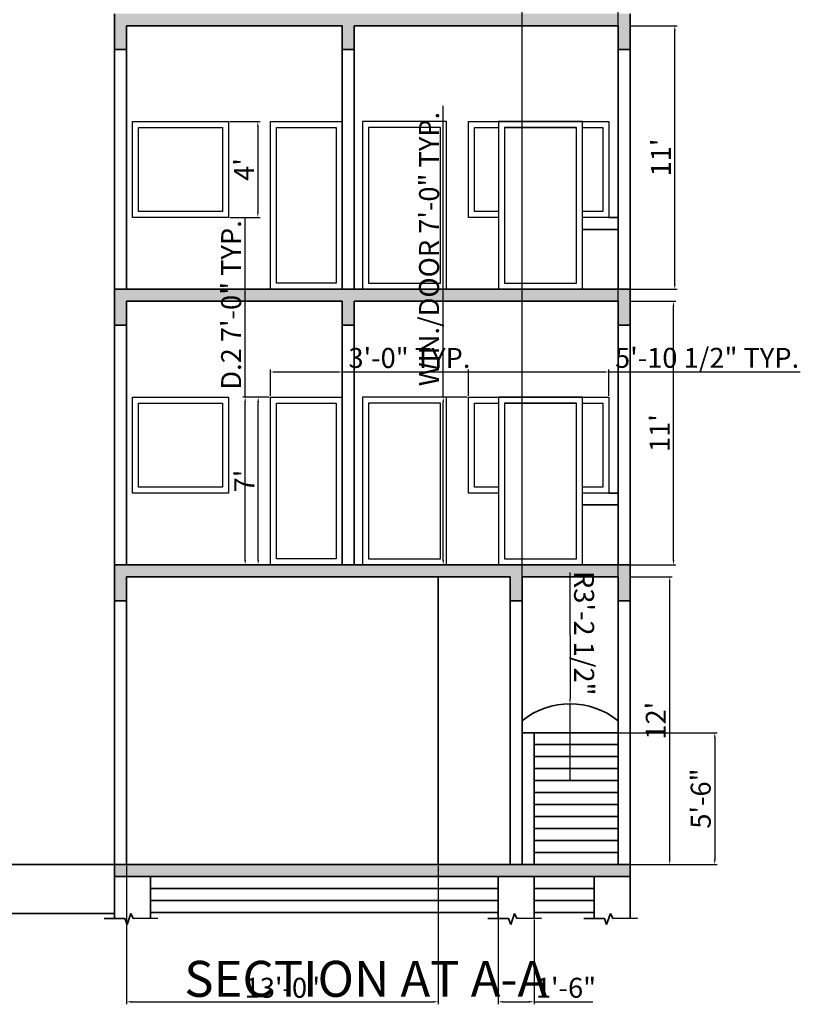
# Model space of a CAD drawing. Units: inches. Extents: x 2368 to 3882, y 1243 to 2139.
# Tile 5 of 6: x 3491 to 3882, y 1252 to 1745. Entities that reach past the tile are written whole.
import ezdxf

# ---------------------------------------------------------------- set-up
doc = ezdxf.new("R2010")
doc.units = ezdxf.units.IN
for name, color, linetype, lineweight in [('A-ANNO-DIMS', 2, 'Continuous', 18), ('A-ANNO-TEXT', 7, 'Continuous', 18), ('A-ELEV', 7, 'Continuous', 25), ('A-SECT', 7, 'Continuous', 35), ('A-SECT-PATT', 8, 'Continuous', 13)]:
    doc.layers.add(name, color=color, linetype=linetype, lineweight=lineweight)
doc.styles.get("Standard").update_dxf_attribs({"font": 'arial.ttf'})
doc.dimstyles.new('ISO-25', dxfattribs={"dimtxt": 10, "dimasz": 2.5, "dimexe": 1.25, "dimexo": 0.625, "dimtad": 1, "dimlunit": 3, "dimtxsty": 'Standard', "dimcen": 2.5, "dimadec": 0, "dimazin": 0, "dimtfac": 1, "dimtmove": 0, "dimatfit": 3, "dimfxl": 1, "dimarcsym": 0})

# ---------------------------------------------------------------- blocks, each defined once
blk = doc.blocks.new('*D8')
at = {"layer": 'A-ANNO-DIMS', "color": 0, "lineweight": -2, "transparency": 16777216}
for p, q in [((3615.71, 1555.84), (3609, 1555.84)), ((3610.25, 1474.34), (3610.25, 1553.34)), ((3615.71, 1471.84), (3609, 1471.84))]:
    blk.add_line(p, q, dxfattribs=at)
at = {"layer": 'A-ANNO-DIMS', "color": 0, "transparency": 16777216}
for points in [[(3609.83, 1553.34), (3610.67, 1553.34), (3610.25, 1555.84)], [(3609.83, 1474.34), (3610.67, 1474.34), (3610.25, 1471.84)]]:
    blk.add_solid(points, dxfattribs=at)
at = {"layer": 'Defpoints', "color": 0, "transparency": 16777216}
for p in [(3610.25, 1555.84), (3616.34, 1555.84), (3616.34, 1471.84)]:
    blk.add_point(p, dxfattribs=at)
at = {"layer": 'A-ANNO-DIMS', "color": 0, "transparency": 16777216, "insert": (3604.62, 1513.84), "char_height": 10, "attachment_point": 5, "rotation": 90}
blk.add_mtext("7'", dxfattribs=at)
blk = doc.blocks.new('*D9')
at = {"layer": 'A-ANNO-DIMS', "color": 0, "lineweight": -2, "transparency": 16777216}
for p, q in [((3596.02, 1693.84), (3611.32, 1693.84)), ((3610.07, 1691.34), (3610.07, 1648.34)), ((3596.02, 1645.84), (3611.32, 1645.84))]:
    blk.add_line(p, q, dxfattribs=at)
at = {"layer": 'A-ANNO-DIMS', "color": 0, "transparency": 16777216}
for points in [[(3609.65, 1691.34), (3610.48, 1691.34), (3610.07, 1693.84)], [(3609.65, 1648.34), (3610.48, 1648.34), (3610.07, 1645.84)]]:
    blk.add_solid(points, dxfattribs=at)
at = {"layer": 'Defpoints', "color": 0, "transparency": 16777216}
for p in [(3595.39, 1693.84), (3595.39, 1645.84), (3610.07, 1645.84)]:
    blk.add_point(p, dxfattribs=at)
at = {"layer": 'A-ANNO-DIMS', "color": 0, "transparency": 16777216, "insert": (3604.44, 1669.84), "char_height": 10, "attachment_point": 5, "rotation": 90}
blk.add_mtext("4'", dxfattribs=at)
blk = doc.blocks.new('*D10')
at = {"layer": 'A-ANNO-DIMS', "color": 0, "lineweight": -2, "transparency": 16777216}
for p, q in [((3796.96, 1465.84), (3817.44, 1465.84)), ((3816.19, 1324.34), (3816.19, 1463.34)), ((3796.96, 1321.84), (3817.44, 1321.84))]:
    blk.add_line(p, q, dxfattribs=at)
at = {"layer": 'A-ANNO-DIMS', "color": 0, "transparency": 16777216}
for points in [[(3815.77, 1463.34), (3816.6, 1463.34), (3816.19, 1465.84)], [(3815.77, 1324.34), (3816.6, 1324.34), (3816.19, 1321.84)]]:
    blk.add_solid(points, dxfattribs=at)
at = {"layer": 'Defpoints', "color": 0, "transparency": 16777216}
for p in [(3796.34, 1465.84), (3816.19, 1465.84), (3796.34, 1321.84)]:
    blk.add_point(p, dxfattribs=at)
at = {"layer": 'A-ANNO-DIMS', "color": 0, "transparency": 16777216, "insert": (3810.54, 1393.84), "char_height": 10, "attachment_point": 5, "rotation": 90}
blk.add_mtext("12'", dxfattribs=at)
blk = doc.blocks.new('*D11')
at = {"layer": 'A-ANNO-DIMS', "color": 0, "lineweight": -2, "transparency": 16777216}
for p, q in [((3796.96, 1603.84), (3819.34, 1603.84)), ((3818.09, 1474.34), (3818.09, 1601.34)), ((3796.96, 1471.84), (3819.34, 1471.84))]:
    blk.add_line(p, q, dxfattribs=at)
at = {"layer": 'A-ANNO-DIMS', "color": 0, "transparency": 16777216}
for points in [[(3817.68, 1601.34), (3818.51, 1601.34), (3818.09, 1603.84)], [(3817.68, 1474.34), (3818.51, 1474.34), (3818.09, 1471.84)]]:
    blk.add_solid(points, dxfattribs=at)
at = {"layer": 'Defpoints', "color": 0, "transparency": 16777216}
for p in [(3796.34, 1603.84), (3818.09, 1603.84), (3796.34, 1471.84)]:
    blk.add_point(p, dxfattribs=at)
at = {"layer": 'A-ANNO-DIMS', "color": 0, "transparency": 16777216, "insert": (3812.45, 1537.84), "char_height": 10, "attachment_point": 5, "rotation": 90}
blk.add_mtext("11'", dxfattribs=at)
blk = doc.blocks.new('*D12')
at = {"layer": 'A-ANNO-DIMS', "color": 0, "lineweight": -2, "transparency": 16777216}
for p, q in [((3796.96, 1741.84), (3819.98, 1741.84)), ((3818.73, 1612.34), (3818.73, 1739.34)), ((3796.96, 1609.84), (3819.98, 1609.84))]:
    blk.add_line(p, q, dxfattribs=at)
at = {"layer": 'A-ANNO-DIMS', "color": 0, "transparency": 16777216}
for points in [[(3818.31, 1739.34), (3819.15, 1739.34), (3818.73, 1741.84)], [(3818.31, 1612.34), (3819.15, 1612.34), (3818.73, 1609.84)]]:
    blk.add_solid(points, dxfattribs=at)
at = {"layer": 'Defpoints', "color": 0, "transparency": 16777216}
for p in [(3796.34, 1741.84), (3818.73, 1741.84), (3796.34, 1609.84)]:
    blk.add_point(p, dxfattribs=at)
at = {"layer": 'A-ANNO-DIMS', "color": 0, "transparency": 16777216, "insert": (3813.09, 1675.84), "char_height": 10, "attachment_point": 5, "rotation": 90}
blk.add_mtext("11'", dxfattribs=at)
blk = doc.blocks.new('WIN-SECT-SQ')
for points in [[(3547.39, 1831.84), (3595.39, 1831.84), (3595.39, 1783.84), (3547.39, 1783.84)], [(3550.39, 1828.84), (3592.39, 1828.84), (3592.39, 1786.84), (3550.39, 1786.84)]]:
    blk.add_lwpolyline(points, close=True)
blk = doc.blocks.new('DOOR-SECT')
for points in [[(3662.52, 1747.84), (3704.52, 1747.84), (3704.52, 1831.84), (3662.52, 1831.84)], [(3665.52, 1750.84), (3701.52, 1750.84), (3701.52, 1828.84), (3665.52, 1828.84)]]:
    blk.add_lwpolyline(points, close=True)
blk = doc.blocks.new('DOOR-SECT-2')
for points in [[(3652.34, 1471.84), (3616.34, 1471.84), (3616.34, 1555.84), (3652.34, 1555.84)], [(3649.34, 1474.84), (3619.34, 1474.84), (3619.34, 1552.84), (3649.34, 1552.84)]]:
    blk.add_lwpolyline(points, close=True)
blk = doc.blocks.new('WIN-DOOR-SECT')
for points in [[(3730.54, 1783.84), (3715.45, 1783.84), (3715.45, 1831.84), (3785.77, 1831.84), (3785.77, 1783.84), (3772.54, 1783.84)], [(3730.54, 1786.84), (3718.45, 1786.84), (3718.45, 1828.84), (3730.54, 1828.84)], [(3733.54, 1828.84), (3769.54, 1828.84)], [(3772.54, 1828.84), (3782.77, 1828.84), (3782.77, 1786.84), (3772.54, 1786.84)]]:
    blk.add_lwpolyline(points)
for points in [[(3730.54, 1747.84), (3772.54, 1747.84), (3772.54, 1831.84), (3730.54, 1831.84)], [(3733.54, 1750.84), (3769.54, 1750.84), (3769.54, 1828.84), (3733.54, 1828.84)]]:
    blk.add_lwpolyline(points, close=True)
blk = doc.blocks.new('*D24')
at = {"layer": 'A-ANNO-DIMS', "color": 0, "lineweight": -2, "transparency": 16777216}
for p, q in [((3702.85, 1555.84), (3702.85, 1701.66)), ((3714.83, 1555.84), (3701.6, 1555.84)), ((3702.85, 1474.34), (3702.85, 1553.34)), ((3714.83, 1471.84), (3701.6, 1471.84))]:
    blk.add_line(p, q, dxfattribs=at)
at = {"layer": 'A-ANNO-DIMS', "color": 0, "transparency": 16777216}
for points in [[(3702.44, 1553.34), (3703.27, 1553.34), (3702.85, 1555.84)], [(3702.44, 1474.34), (3703.27, 1474.34), (3702.85, 1471.84)]]:
    blk.add_solid(points, dxfattribs=at)
at = {"layer": 'Defpoints', "color": 0, "transparency": 16777216}
for p in [(3702.85, 1555.84), (3715.45, 1555.84), (3715.45, 1471.84)]:
    blk.add_point(p, dxfattribs=at)
at = {"layer": 'A-ANNO-DIMS', "color": 0, "transparency": 16777216, "insert": (3697.06, 1630), "char_height": 10, "attachment_point": 5, "rotation": 90}
blk.add_mtext('WIN./DOOR 7\'-0" TYP.', dxfattribs=at)
blk = doc.blocks.new('*D25')
at = {"layer": 'A-ANNO-DIMS', "color": 0, "lineweight": -2, "transparency": 16777216}
for p, q in [((3715.45, 1556.46), (3715.45, 1569.69)), ((3717.95, 1568.44), (3783.27, 1568.44)), ((3785.77, 1556.46), (3785.77, 1569.69)), ((3785.77, 1568.44), (3881.55, 1568.44))]:
    blk.add_line(p, q, dxfattribs=at)
at = {"layer": 'A-ANNO-DIMS', "color": 0, "transparency": 16777216}
for points in [[(3717.95, 1568.85), (3717.95, 1568.02), (3715.45, 1568.44)], [(3783.27, 1568.85), (3783.27, 1568.02), (3785.77, 1568.44)]]:
    blk.add_solid(points, dxfattribs=at)
at = {"layer": 'Defpoints', "color": 0, "transparency": 16777216}
for p in [(3785.77, 1568.44), (3715.45, 1555.84), (3785.77, 1555.84)]:
    blk.add_point(p, dxfattribs=at)
at = {"layer": 'A-ANNO-DIMS', "color": 0, "transparency": 16777216, "insert": (3834.91, 1574.23), "char_height": 10, "attachment_point": 5}
blk.add_mtext('5\'-10 1/2" TYP.', dxfattribs=at)
blk = doc.blocks.new('*D30')
at = {"layer": 'A-ANNO-DIMS', "color": 0, "lineweight": -2, "transparency": 16777216}
for p, q in [((3603.74, 1555.84), (3603.74, 1645.67)), ((3615.71, 1555.84), (3602.49, 1555.84)), ((3603.74, 1474.34), (3603.74, 1553.34)), ((3615.71, 1471.84), (3602.49, 1471.84))]:
    blk.add_line(p, q, dxfattribs=at)
at = {"layer": 'A-ANNO-DIMS', "color": 0, "transparency": 16777216}
for points in [[(3603.32, 1553.34), (3604.15, 1553.34), (3603.74, 1555.84)], [(3603.32, 1474.34), (3604.15, 1474.34), (3603.74, 1471.84)]]:
    blk.add_solid(points, dxfattribs=at)
at = {"layer": 'Defpoints', "color": 0, "transparency": 16777216}
for p in [(3603.74, 1555.84), (3616.34, 1555.84), (3616.34, 1471.84)]:
    blk.add_point(p, dxfattribs=at)
at = {"layer": 'A-ANNO-DIMS', "color": 0, "transparency": 16777216, "insert": (3598.01, 1602), "char_height": 10, "attachment_point": 5, "rotation": 90}
blk.add_mtext('D.2 7\'-0" TYP.', dxfattribs=at)
blk = doc.blocks.new('*D31')
at = {"layer": 'A-ANNO-DIMS', "color": 0, "lineweight": -2, "transparency": 16777216}
for p, q in [((3616.34, 1556.46), (3616.34, 1569.69)), ((3618.84, 1568.44), (3649.84, 1568.44)), ((3652.34, 1556.46), (3652.34, 1569.69)), ((3652.34, 1568.44), (3717.04, 1568.44))]:
    blk.add_line(p, q, dxfattribs=at)
at = {"layer": 'A-ANNO-DIMS', "color": 0, "transparency": 16777216}
for points in [[(3618.84, 1568.85), (3618.84, 1568.02), (3616.34, 1568.44)], [(3649.84, 1568.85), (3649.84, 1568.02), (3652.34, 1568.44)]]:
    blk.add_solid(points, dxfattribs=at)
at = {"layer": 'Defpoints', "color": 0, "transparency": 16777216}
for p in [(3652.34, 1568.44), (3616.34, 1555.84), (3652.34, 1555.84)]:
    blk.add_point(p, dxfattribs=at)
at = {"layer": 'A-ANNO-DIMS', "color": 0, "transparency": 16777216, "insert": (3685.94, 1574.17), "char_height": 10, "attachment_point": 5}
blk.add_mtext('3\'-0" TYP.', dxfattribs=at)
blk = doc.blocks.new('*D92')
at = {"layer": 'A-ANNO-DIMS', "color": 0, "lineweight": -2, "transparency": 16777216}
for p, q in [((3380.64, 1321.84), (3380.64, 1375.64)), ((3537.71, 1321.84), (3379.39, 1321.84)), ((3380.64, 1299.76), (3380.64, 1319.34)), ((3537.71, 1297.26), (3379.39, 1297.26))]:
    blk.add_line(p, q, dxfattribs=at)
at = {"layer": 'A-ANNO-DIMS', "color": 0, "transparency": 16777216}
for points in [[(3380.23, 1319.34), (3381.06, 1319.34), (3380.64, 1321.84)], [(3380.23, 1299.76), (3381.06, 1299.76), (3380.64, 1297.26)]]:
    blk.add_solid(points, dxfattribs=at)
at = {"layer": 'Defpoints', "color": 0, "transparency": 16777216}
for p in [(3380.64, 1321.84), (3538.34, 1321.84), (3538.34, 1297.26)]:
    blk.add_point(p, dxfattribs=at)
at = {"layer": 'A-ANNO-DIMS', "color": 0, "transparency": 16777216, "insert": (3374.85, 1349.99), "char_height": 10, "attachment_point": 5, "rotation": 90}
blk.add_mtext('2\'-0 1/2"', dxfattribs=at)
blk = doc.blocks.new('*D93')
at = {"layer": 'A-ANNO-DIMS', "color": 0, "lineweight": -2, "transparency": 16777216}
for p, q in [((3730.34, 1294.21), (3730.34, 1251.83)), ((3748.34, 1294.21), (3748.34, 1251.83)), ((3732.84, 1253.08), (3745.84, 1253.08)), ((3748.34, 1253.08), (3777.73, 1253.08))]:
    blk.add_line(p, q, dxfattribs=at)
at = {"layer": 'A-ANNO-DIMS', "color": 0, "transparency": 16777216}
for points in [[(3732.84, 1253.49), (3732.84, 1252.66), (3730.34, 1253.08)], [(3745.84, 1253.49), (3745.84, 1252.66), (3748.34, 1253.08)]]:
    blk.add_solid(points, dxfattribs=at)
at = {"layer": 'Defpoints', "color": 0, "transparency": 16777216}
for p in [(3730.34, 1294.84), (3748.34, 1294.84), (3748.34, 1253.08)]:
    blk.add_point(p, dxfattribs=at)
at = {"layer": 'A-ANNO-DIMS', "color": 0, "transparency": 16777216, "insert": (3764.28, 1258.81), "char_height": 10, "attachment_point": 5}
blk.add_mtext('1\'-6"', dxfattribs=at)
blk = doc.blocks.new('*D94')
at = {"layer": 'A-ANNO-DIMS', "color": 0, "lineweight": -2, "transparency": 16777216}
for p, q in [((3742.34, 1388.46), (3742.34, 2045.79)), ((3744.84, 2044.54), (3787.84, 2044.54)), ((3790.34, 1388.46), (3790.34, 2045.79))]:
    blk.add_line(p, q, dxfattribs=at)
at = {"layer": 'A-ANNO-DIMS', "color": 0, "transparency": 16777216}
for points in [[(3744.84, 2044.95), (3744.84, 2044.12), (3742.34, 2044.54)], [(3787.84, 2044.95), (3787.84, 2044.12), (3790.34, 2044.54)]]:
    blk.add_solid(points, dxfattribs=at)
at = {"layer": 'Defpoints', "color": 0, "transparency": 16777216}
for p in [(3790.34, 2044.54), (3742.34, 1387.84), (3790.34, 1387.84)]:
    blk.add_point(p, dxfattribs=at)
at = {"layer": 'A-ANNO-DIMS', "color": 0, "transparency": 16777216, "insert": (3766.34, 2050.27), "char_height": 10, "attachment_point": 5}
blk.add_mtext('4\'-0"', dxfattribs=at)
blk = doc.blocks.new('*D95')
at = {"layer": 'A-ANNO-DIMS', "color": 0, "lineweight": -2, "transparency": 16777216}
for p, q in [((3790.96, 1387.84), (3839.99, 1387.84)), ((3838.74, 1385.34), (3838.74, 1324.34)), ((3790.96, 1321.84), (3839.99, 1321.84))]:
    blk.add_line(p, q, dxfattribs=at)
at = {"layer": 'A-ANNO-DIMS', "color": 0, "transparency": 16777216}
for points in [[(3838.33, 1385.34), (3839.16, 1385.34), (3838.74, 1387.84)], [(3838.33, 1324.34), (3839.16, 1324.34), (3838.74, 1321.84)]]:
    blk.add_solid(points, dxfattribs=at)
at = {"layer": 'Defpoints', "color": 0, "transparency": 16777216}
for p in [(3790.34, 1387.84), (3790.34, 1321.84), (3838.74, 1321.84)]:
    blk.add_point(p, dxfattribs=at)
at = {"layer": 'A-ANNO-DIMS', "color": 0, "transparency": 16777216, "insert": (3833.01, 1354.84), "char_height": 10, "attachment_point": 5, "rotation": 90}
blk.add_mtext('5\'-6"', dxfattribs=at)
blk = doc.blocks.new('*D96')
at = {"layer": 'A-ANNO-DIMS', "color": 0, "lineweight": -2, "transparency": 16777216}
for p, q in [((3544.34, 1321.21), (3544.34, 1251.83)), ((3700.34, 1321.21), (3700.34, 1251.83)), ((3546.84, 1253.08), (3697.84, 1253.08))]:
    blk.add_line(p, q, dxfattribs=at)
at = {"layer": 'A-ANNO-DIMS', "color": 0, "transparency": 16777216}
for points in [[(3546.84, 1253.49), (3546.84, 1252.66), (3544.34, 1253.08)], [(3697.84, 1253.49), (3697.84, 1252.66), (3700.34, 1253.08)]]:
    blk.add_solid(points, dxfattribs=at)
at = {"layer": 'Defpoints', "color": 0, "transparency": 16777216}
for p in [(3544.34, 1321.84), (3700.34, 1321.84), (3700.34, 1253.08)]:
    blk.add_point(p, dxfattribs=at)
at = {"layer": 'A-ANNO-DIMS', "color": 0, "transparency": 16777216, "insert": (3622.34, 1258.81), "char_height": 10, "attachment_point": 5}
blk.add_mtext('13\'-0"', dxfattribs=at)
blk = doc.blocks.new('*D98')
at = {"layer": 'A-ANNO-DIMS', "color": 0, "lineweight": -2, "transparency": 16777216}
for p, q in [((3766.24, 1467.96), (3766.3, 1404.76)), ((3766.34, 1363.84), (3766.3, 1402.26))]:
    blk.add_line(p, q, dxfattribs=at)
at = {"layer": 'A-ANNO-DIMS', "color": 0, "transparency": 16777216}
blk.add_solid([(3766.71, 1404.76), (3765.88, 1404.76), (3766.3, 1402.26)], dxfattribs=at)
at = {"layer": 'Defpoints', "color": 0, "transparency": 16777216}
for p in [(3766.3, 1402.26), (3766.34, 1363.84)]:
    blk.add_point(p, dxfattribs=at)
at = {"layer": 'A-ANNO-DIMS', "color": 0, "transparency": 16777216, "insert": (3772.06, 1437.61), "char_height": 10, "attachment_point": 5, "rotation": 270.0563}
blk.add_mtext('R3\'-2 1/2"', dxfattribs=at)

msp = doc.modelspace()

# ---------------------------------------------------------------- hatches: boundary and pattern name
at = {"layer": 'A-SECT-PATT'}
h = msp.add_hatch(color=256, dxfattribs=at)
h.dxf.hatch_style = 1
h.paths.add_polyline_path([(3796.338, 1321.838), (3538.338, 1321.838), (3538.338, 1315.838), (3796.338, 1315.838)])
h.paths.add_polyline_path([(3796.338, 1471.838), (3538.338, 1471.838), (3538.338, 1453.838), (3544.338, 1453.838), (3544.338, 1465.838), (3736.338, 1465.838), (3736.338, 1453.838), (3742.338, 1453.838), (3742.338, 1465.838), (3790.338, 1465.838), (3790.338, 1453.838), (3796.338, 1453.838), (3796.338, 1465.838)])
h.paths.add_polyline_path([(3796.338, 1609.838), (3538.338, 1609.838), (3538.338, 1591.838), (3544.338, 1591.838), (3544.338, 1603.838), (3652.338, 1603.838), (3652.338, 1591.838), (3658.338, 1591.838), (3658.338, 1603.838), (3790.338, 1603.838), (3790.338, 1591.838), (3796.338, 1591.838), (3796.338, 1603.838)])
h.paths.add_polyline_path([(3796.338, 1747.838), (3538.338, 1747.838), (3538.338, 1729.838), (3544.338, 1729.838), (3544.338, 1741.838), (3652.338, 1741.838), (3652.338, 1729.838), (3658.338, 1729.838), (3658.338, 1741.838), (3790.338, 1741.838), (3790.338, 1729.838), (3796.338, 1729.838), (3796.338, 1741.838)])
h.paths.add_polyline_path([(3796.338, 1885.838), (3538.338, 1885.838), (3538.338, 1867.838), (3544.338, 1867.838), (3544.338, 1879.838), (3652.338, 1879.838), (3652.338, 1867.838), (3658.338, 1867.838), (3658.338, 1879.838), (3790.338, 1879.838), (3790.338, 1867.838), (3796.338, 1867.838), (3796.338, 1879.838)])

# ---------------------------------------------------------------- linework, layer by layer
at = {"layer": 'A-SECT'}
for p, q in [((3538.338, 1609.838), (3538.338, 1747.838)), ((3796.338, 1741.838), (3796.338, 1747.838)), ((3544.338, 1741.838), (3652.338, 1741.838)), ((3544.338, 1609.838), (3544.338, 1741.838)), ((3652.338, 1609.838), (3652.338, 1741.838)), ((3658.338, 1609.838), (3658.338, 1741.838)), ((3658.338, 1741.838), (3790.338, 1741.838)), ((3790.338, 1609.838), (3790.338, 1741.838)), ((3796.338, 1609.838), (3796.338, 1741.838)), ((3544.338, 1729.838), (3538.338, 1729.838)), ((3658.338, 1729.838), (3652.338, 1729.838)), ((3796.338, 1729.838), (3790.338, 1729.838)), ((3785.773, 1645.838), (3790.338, 1645.838)), ((3772.538, 1639.838), (3790.338, 1639.838)), ((3538.338, 1471.838), (3538.338, 1609.838)), ((3796.338, 1609.838), (3538.338, 1609.838)), ((3796.338, 1603.838), (3796.338, 1609.838)), ((3544.338, 1603.838), (3652.338, 1603.838)), ((3544.338, 1471.838), (3544.338, 1603.838)), ((3652.338, 1471.838), (3652.338, 1603.838)), ((3658.338, 1471.838), (3658.338, 1603.838)), ((3658.338, 1603.838), (3790.338, 1603.838)), ((3790.338, 1471.838), (3790.338, 1603.838)), ((3796.338, 1471.838), (3796.338, 1603.838)), ((3544.338, 1591.838), (3538.338, 1591.838)), ((3658.338, 1591.838), (3652.338, 1591.838)), ((3796.338, 1591.838), (3790.338, 1591.838)), ((3785.773, 1507.838), (3790.338, 1507.838)), ((3772.538, 1501.838), (3790.338, 1501.838)), ((3538.338, 1294.838), (3538.338, 1471.838)), ((3796.338, 1471.838), (3538.338, 1471.838)), ((3796.338, 1465.838), (3796.338, 1471.838)), ((3544.338, 1465.838), (3736.338, 1465.838)), ((3544.338, 1321.838), (3544.338, 1465.838)), ((3700.338, 1321.838), (3700.338, 1465.838)), ((3736.338, 1321.838), (3736.338, 1465.838)), ((3742.338, 1321.838), (3742.338, 1465.838)), ((3742.338, 1465.838), (3790.338, 1465.838)), ((3790.338, 1321.838), (3790.338, 1465.838)), ((3796.338, 1321.838), (3796.338, 1465.838)), ((3544.338, 1453.838), (3538.338, 1453.838)), ((3742.338, 1453.838), (3736.338, 1453.838)), ((3796.338, 1453.838), (3790.338, 1453.838)), ((3790.338, 1387.838), (3742.338, 1387.838)), ((3748.338, 1321.838), (3748.338, 1387.838)), ((3790.338, 1381.838), (3748.338, 1381.838)), ((3790.338, 1375.838), (3748.338, 1375.838)), ((3790.338, 1369.838), (3748.338, 1369.838)), ((3790.338, 1363.838), (3748.338, 1363.838)), ((3790.338, 1357.838), (3748.338, 1357.838)), ((3790.338, 1351.838), (3748.338, 1351.838)), ((3790.338, 1345.838), (3748.338, 1345.838)), ((3790.338, 1339.838), (3748.338, 1339.838)), ((3790.338, 1333.838), (3748.338, 1333.838)), ((3790.338, 1327.838), (3748.338, 1327.838)), ((3538.338, 1321.838), (3419.342, 1321.838)), ((3796.338, 1321.838), (3538.338, 1321.838)), ((3790.338, 1321.838), (3742.338, 1321.838)), ((3796.338, 1294.838), (3796.338, 1321.838)), ((3796.338, 1315.838), (3538.338, 1315.838)), ((3556.338, 1294.838), (3556.338, 1315.838)), ((3730.338, 1294.838), (3730.338, 1315.838)), ((3748.338, 1294.838), (3748.338, 1315.838)), ((3778.338, 1294.838), (3778.338, 1315.838)), ((3730.338, 1309.838), (3556.338, 1309.838)), ((3778.338, 1309.838), (3748.338, 1309.838)), ((3730.338, 1303.838), (3556.338, 1303.838)), ((3778.338, 1303.838), (3748.338, 1303.838)), ((3538.338, 1297.261), (3420.08, 1297.261)), ((3544.63, 1291.775), (3546.535, 1297.313)), ((3546.535, 1297.313), (3547.712, 1294.838)), ((3556.338, 1297.838), (3730.338, 1297.838)), ((3736.63, 1291.775), (3738.535, 1297.313)), ((3738.535, 1297.313), (3739.712, 1294.838)), ((3748.338, 1297.838), (3778.338, 1297.838)), ((3784.63, 1291.775), (3786.535, 1297.313)), ((3786.535, 1297.313), (3787.712, 1294.838)), ((3533.199, 1294.838), (3543.486, 1294.838)), ((3543.486, 1294.838), (3544.63, 1291.775)), ((3547.712, 1294.838), (3560.044, 1294.89)), ((3725.199, 1294.838), (3735.486, 1294.838)), ((3735.486, 1294.838), (3736.63, 1291.775)), ((3739.712, 1294.838), (3752.044, 1294.89)), ((3773.199, 1294.838), (3783.486, 1294.838)), ((3783.486, 1294.838), (3784.63, 1291.775)), ((3787.712, 1294.838), (3800.044, 1294.89))]:
    msp.add_line(p, q, dxfattribs=at)
msp.add_arc((3766.338, 1363.838), 38.419, 51.34019, 128.65981, dxfattribs=at)

# ---------------------------------------------------------------- block references
at = {"layer": 'A-ELEV'}
for name, p in [('WIN-SECT-SQ', (0, -138)), ('DOOR-SECT-2', (0, 138)), ('DOOR-SECT', (0, -138)), ('WIN-DOOR-SECT', (0, -138)), ('WIN-SECT-SQ', (0, -276)), ('DOOR-SECT-2', (0, 0)), ('DOOR-SECT', (0, -276)), ('WIN-DOOR-SECT', (0, -276))]:
    msp.add_blockref(name, p, dxfattribs=at)

# ---------------------------------------------------------------- texts
at = {"layer": 'A-ANNO-TEXT'}
msp.add_text('SECTION AT A-A', height=18, dxfattribs=at).set_placement((3573.285, 1255.58))

# ---------------------------------------------------------------- dimensions: what is measured, and where the dimension line sits
at = {"layer": 'A-ANNO-DIMS'}
for base, p1, p2, picture, middle in [((3790.338, 2044.538), (3742.338, 1387.838), (3790.338, 1387.838), '*D94', (3766.338, 2050.268)), ((3700.338, 1253.075), (3544.338, 1321.838), (3700.338, 1321.838), '*D96', (3622.338, 1258.809)), ((3748.338, 1253.075), (3730.338, 1294.838), (3748.338, 1294.838), '*D93', (3764.283, 1258.806))]:
    dim = msp.add_linear_dim(base=base, p1=p1, p2=p2, dimstyle='ISO-25', override={"dimdec": 1, "dimlfac": 1, "dimrnd": 0, "dimzin": 1, "dimdsep": 46, "dimlunit": 4, "dimfrac": 2}, dxfattribs=at)
    dim.commit()
    dim.dimension.update_dxf_attribs({"geometry": picture, "text_midpoint": middle})
for base, p1, p2, override, picture, middle in [((3818.731, 1741.838), (3796.338, 1609.838), (3796.338, 1741.838), {"dimclrd": 0, "dimclre": 0, "dimclrt": 0}, '*D12', (3813.086, 1675.838)), ((3610.065, 1645.838), (3595.393, 1693.838), (3595.393, 1645.838), {"dimclrd": 0, "dimclre": 0, "dimclrt": 0}, '*D9', (3604.44, 1669.838)), ((3818.095, 1603.838), (3796.338, 1471.838), (3796.338, 1603.838), {"dimclrd": 0, "dimclre": 0, "dimclrt": 0}, '*D11', (3812.449, 1537.838)), ((3610.25, 1555.838), (3616.338, 1471.838), (3616.338, 1555.838), {"dimclrd": 0, "dimclre": 0, "dimclrt": 0}, '*D8', (3604.625, 1513.838)), ((3816.188, 1465.838), (3796.338, 1321.838), (3796.338, 1465.838), {"dimclrd": 0, "dimclre": 0, "dimclrt": 0}, '*D10', (3810.543, 1393.838)), ((3838.744, 1321.838), (3790.338, 1387.838), (3790.338, 1321.838), {"dimdec": 1, "dimlfac": 1, "dimrnd": 0, "dimzin": 1, "dimdsep": 46, "dimlunit": 4, "dimfrac": 2}, '*D95', (3833.013, 1354.838)), ((3380.642, 1321.838), (3538.338, 1297.261), (3538.338, 1321.838), {"dimdec": 1, "dimlfac": 1, "dimrnd": 0, "dimzin": 1, "dimdsep": 46, "dimlunit": 4, "dimfrac": 2}, '*D92', (3374.847, 1349.99))]:
    dim = msp.add_linear_dim(base=base, p1=p1, p2=p2, angle=90, dimstyle='ISO-25', override=override, dxfattribs=at)
    dim.commit()
    dim.dimension.update_dxf_attribs({"geometry": picture, "text_midpoint": middle})
for base, p1, p2, text, picture, middle in [((3702.854, 1555.838), (3715.454, 1471.838), (3715.454, 1555.838), 'WIN./DOOR <> TYP.', '*D24', (3697.055, 1629.999)), ((3603.738, 1555.838), (3616.338, 1471.838), (3616.338, 1555.838), 'D.2 <> TYP.', '*D30', (3598.007, 1602.002))]:
    dim = msp.add_linear_dim(base=base, p1=p1, p2=p2, angle=90, text=text, dimstyle='ISO-25', override={"dimdec": 1, "dimrnd": 0, "dimzin": 1, "dimlunit": 4, "dimfrac": 2}, dxfattribs=at)
    dim.commit()
    dim.dimension.update_dxf_attribs({"geometry": picture, "text_midpoint": middle})
for base, p1, p2, picture, middle in [((3785.773, 1568.438), (3715.454, 1555.838), (3785.773, 1555.838), '*D25', (3834.911, 1574.233)), ((3652.338, 1568.438), (3616.338, 1555.838), (3652.338, 1555.838), '*D31', (3685.937, 1574.172))]:
    dim = msp.add_linear_dim(base=base, p1=p1, p2=p2, text='<> TYP.', dimstyle='ISO-25', override={"dimdec": 1, "dimrnd": 0, "dimzin": 1, "dimlunit": 4, "dimfrac": 2}, dxfattribs=at)
    dim.commit()
    dim.dimension.update_dxf_attribs({"geometry": picture, "text_midpoint": middle})
dim = msp.add_radius_dim(center=(3766.338, 1363.838), mpoint=(3766.3, 1402.256), dimstyle='ISO-25', override={"dimdec": 1, "dimlfac": 1, "dimrnd": 0, "dimzin": 1, "dimdsep": 46, "dimlunit": 4, "dimfrac": 2}, dxfattribs=at)
dim.commit()
dim.dimension.update_dxf_attribs({"geometry": '*D98', "text_midpoint": (3772.064, 1437.614)})

doc.saveas('drawing.dxf')
